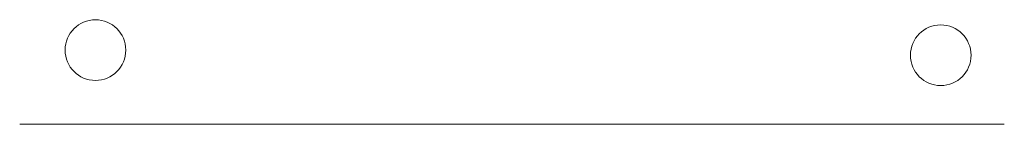
# Model space of a CAD drawing. Units: millimetres. Extents: x 214.3 to 279.3, y 0 to 47.9.
# Tile 1 of 1: x 214.28 to 279.28, y 0 to 6.89. Entities that reach past the tile are written whole.
import ezdxf

# ---------------------------------------------------------------- set-up
doc = ezdxf.new("R2010")
doc.units = ezdxf.units.MM
doc.layers.add('M-CONS', color=8, linetype='Continuous', lineweight=18)

msp = doc.modelspace()

# ---------------------------------------------------------------- linework, layer by layer
at = {"layer": 'M-CONS', "extrusion": (0, -1, 0)}
msp.add_line((214.285, 0, 102.809), (214.285, 0, 96.809), dxfattribs=at)
msp.add_lwpolyline([(214.285, 111.809), (224.285, 111.809), (224.285, 104.809, 0.414214), (226.285, 102.809), (236.539, 102.809, 0.341999), (238.475, 104.309, -0.774597), (250.094, 104.309, 0.341999), (252.031, 102.809), (279.285, 102.809), (279.285, 96.809), (214.285, 96.809)], format="xyb", close=True, dxfattribs=at)
at = {"layer": 'M-CONS'}
for centre in [(219.285, 4.885, 111.809), (275.089, 4.548)]:
    msp.add_circle(centre, 2, dxfattribs=at)
at = {"layer": 'M-CONS', "extrusion": (0, -1, 0)}
msp.add_circle((244.285, 102.809), 2, dxfattribs=at)
msp.add_circle((244.285, 102.809), 2, dxfattribs=at)

doc.saveas('drawing.dxf')
